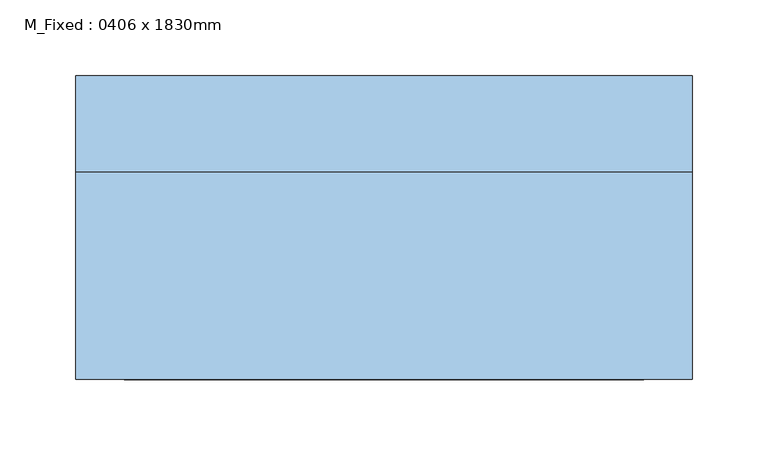
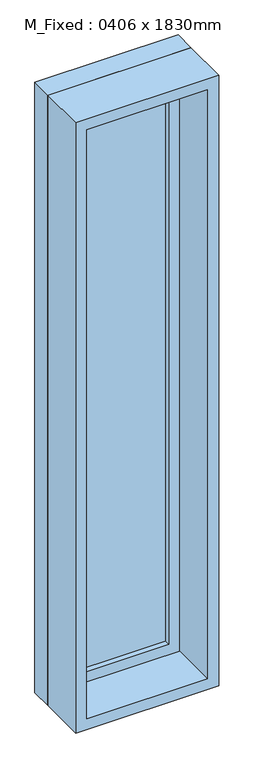
"""IFC4 building model written with IfcOpenShell, lengths in millimetres: window geometry, M_Fixed : 0406 x 1830mm."""

from ifc_helpers import new_model, si_unit, frame, origin, place, context, project, spatial, polyline, outline, extrude, source, transform, mapped, element, save


def m_fixed_0406_x_1830mm_fda39e01(model_context):
    return source(origin(), model_context, "Body", "SweptSolid", [
        extrude(outline(polyline([(-140.0, 78.0), (140.0, 78.0), (140.0, 66.0), (-140.0, 66.0), (-140.0, 78.0)])), frame((0.0, 0.0, 368.0), z_axis=(0.0, 0.0, 1.0), x_axis=(1.0, 0.0, 0.0)), (0.0, 0.0, 1.0), 1704.0),
        extrude(outline(polyline([(2116.0, -184.0), (324.0, -184.0), (324.0, 184.0), (2116.0, 184.0), (2116.0, -184.0)]), holes=[polyline([(2072.0, -140.0), (2072.0, 140.0), (368.0, 140.0), (368.0, -140.0), (2072.0, -140.0)])]), frame((0.0, 50.0, 0.0), z_axis=(0.0, 1.0, 0.0), x_axis=(0.0, 0.0, 1.0)), (0.0, 0.0, 1.0), 44.0),
        extrude(outline(polyline([(2135.0, -203.0), (305.0, -203.0), (305.0, 203.0), (2135.0, 203.0), (2135.0, -203.0)]), holes=[polyline([(2116.0, -184.0), (2116.0, 184.0), (324.0, 184.0), (324.0, -184.0), (2116.0, -184.0)])]), frame((0.0, 50.0, 0.0), z_axis=(0.0, 1.0, 0.0), x_axis=(0.0, 0.0, 1.0)), (0.0, 0.0, 1.0), 63.0),
        extrude(outline(polyline([(2135.0, -203.0), (305.0, -203.0), (305.0, 203.0), (2135.0, 203.0), (2135.0, -203.0)]), holes=[polyline([(2103.0, -171.0), (2103.0, 171.0), (337.0, 171.0), (337.0, -171.0), (2103.0, -171.0)])]), frame((0.0, -87.0, 0.0), z_axis=(0.0, 1.0, 0.0), x_axis=(0.0, 0.0, 1.0)), (0.0, 0.0, 1.0), 137.0),
    ])


if __name__ == "__main__":
    model = new_model("IFC4")
    model_context = context("Model", 3, world=origin())
    ifc_project = project(units=[si_unit("LENGTHUNIT", "METRE", prefix="MILLI")], contexts=[model_context])
    site = spatial("IfcSite", under=ifc_project)
    building = spatial("IfcBuilding", under=site)
    placement = place(None, origin())
    m_fixed_0406_x_1830mm_shape = m_fixed_0406_x_1830mm_fda39e01(model_context)
    element("IfcWindow", 1, ObjectType="M_Fixed : 0406 x 1830mm", at=placement, inside=building, context=model_context, shape_type="MappedRepresentation", body=[
        mapped(m_fixed_0406_x_1830mm_shape, transform((0.0, 0.0, 0.0), x_axis=(1.0, 0.0, 0.0), y_axis=(0.0, 1.0, 0.0), z_axis=(0.0, 0.0, 1.0))),
    ])
    save(model, "model.ifc")

# Revit data of these elements
# Type "M_Fixed : 0406 x 1830mm"
#   Type Mark = "16"
#   Height = 6' - 0.04724"
#   Default Sill Height = 1' - 0.00787"
#   Width = 1' - 3.98425"
#   Window Inset = 0' - 0.74803"
#   Frame Exterior Material = Sash
#   Frame Interior Material = Sash
#   Glass Pane Material = Glass
#   Sash = Sash
#   Wall Closure = (empty or 0)
# Element 1 (IfcWindow, "M_Fixed : 0406 x 1830mm")
#   Materials on its faces: "Sash", "Glass"
# Materials
#   "Sash": class "Wood", colour RGB 136 99 55, transparency 0
#   "Glass": class "Glass", colour RGB 218 227 224, transparency 0.85, Description = "Soda Lime Glass", Cost = 0
